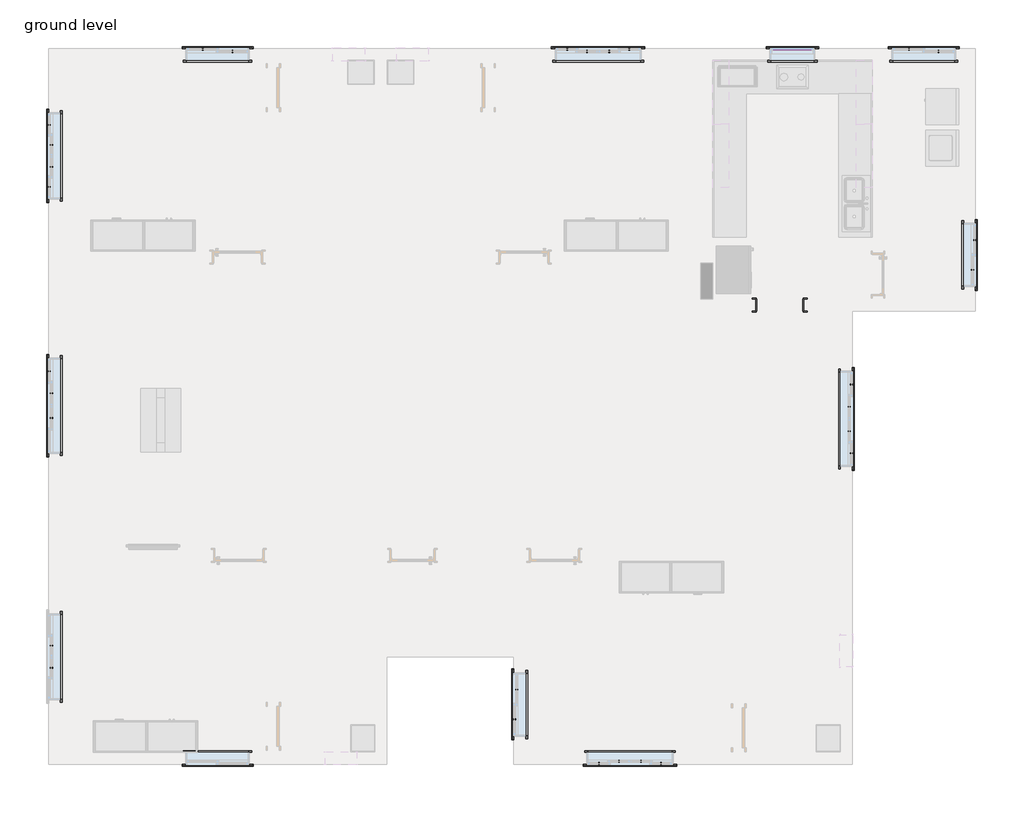
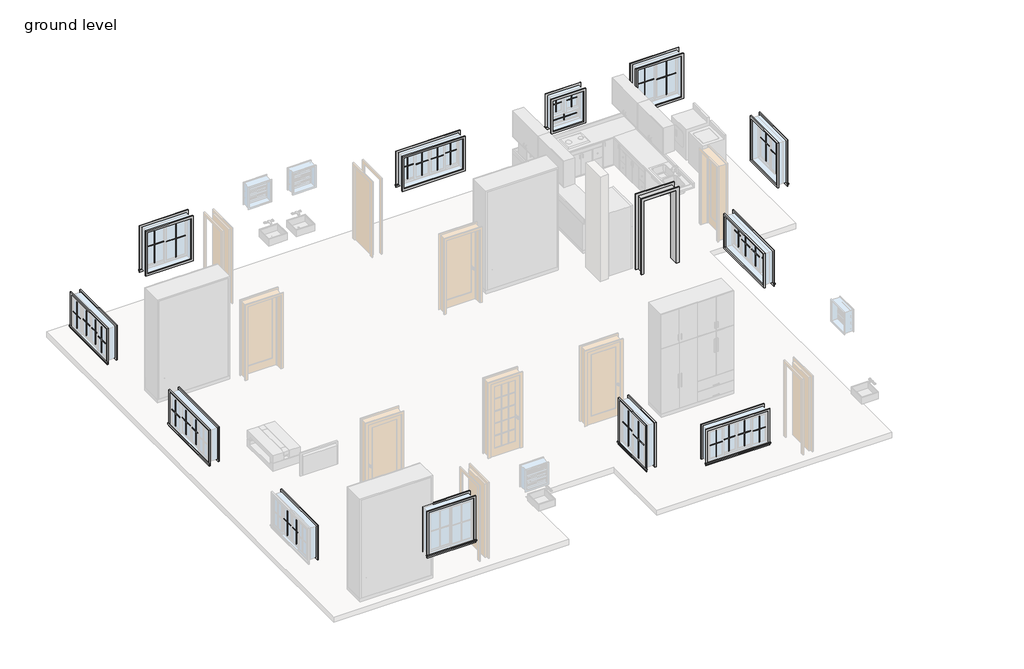
# One storey, part 2 of 2: 56 proxies.
"""IFC4 building model written with IfcOpenShell, lengths in millimetres."""

from ifc_helpers import new_model, si_unit, origin, place, context, project, spatial, transform, mapped, element, save
from components import muntin_pattern_2x2_muntin_pattern_2x2_6186d23a, muntin_pattern_2x2_muntin_pattern_2x2_31a16349, muntin_pattern_2x2_muntin_pattern_2x2_cf37b409, muntin_pattern_2x2_muntin_pattern_2x2_78ce0566, muntin_pattern_2x2_muntin_pattern_2x2_27bf4e5b, muntin_pattern_2x2_muntin_pattern_2x2_8320156c, proxy_e9bf662a, trim_window_exterior_flat_with_sill_c3f87112, trim_window_exterior_flat_with_sill_3c945769, trim_window_exterior_flat_with_sill_7cfdd449, trim_window_exterior_flat_with_sill_41619996, trim_window_interior_flat_picture_frame_1c33fa8a, trim_window_interior_flat_picture_frame_0edfbaa2, trim_window_interior_flat_picture_frame_f1e0b15b, trim_window_interior_flat_picture_frame_51c85655

model = new_model("IFC4")

# Units and contexts
model_context = context("Model", 3, world=origin())
ifc_project = project(units=[si_unit("LENGTHUNIT", "METRE", prefix="MILLI")], contexts=[model_context])

# Site, building, storey
site = spatial("IfcSite", under=ifc_project)
building = spatial("IfcBuilding", under=site)
storey = spatial("IfcBuildingStorey", under=building, Name="ground level", Elevation=609.6)

# Proxies
placement = place(None, origin())
muntin_pattern_2x2_muntin_pattern_2x2_shape = muntin_pattern_2x2_muntin_pattern_2x2_6186d23a(model_context)
element("IfcBuildingElementProxy", 1, Name="Muntin Pattern_2x2 : Muntin Pattern_2x2", ObjectType="Muntin Pattern_2x2 : Muntin Pattern_2x2", at=placement, inside=storey, context=model_context, shape_type="MappedRepresentation", body=[
    mapped(muntin_pattern_2x2_muntin_pattern_2x2_shape, transform((1905.0010838, 7064.4410813, 1606.55), x_axis=(1.0, 0.0, 0.0), y_axis=(0.0, 1.0, 0.0), z_axis=(0.0, 0.0, 1.0))),
])
element("IfcBuildingElementProxy", 2, Name="Muntin Pattern_2x2 : Muntin Pattern_2x2", ObjectType="Muntin Pattern_2x2 : Muntin Pattern_2x2", at=placement, inside=storey, context=model_context, shape_type="MappedRepresentation", body=[
    mapped(muntin_pattern_2x2_muntin_pattern_2x2_shape, transform((2286.0010838, 7019.9910813, 1606.55), x_axis=(1.0, 0.0, 0.0), y_axis=(0.0, 1.0, 0.0), z_axis=(0.0, 0.0, 1.0))),
])
element("IfcBuildingElementProxy", 3, Name="Muntin Pattern_2x2 : Muntin Pattern_2x2", ObjectType="Muntin Pattern_2x2 : Muntin Pattern_2x2", at=placement, inside=storey, context=model_context, shape_type="MappedRepresentation", body=[
    mapped(muntin_pattern_2x2_muntin_pattern_2x2_shape, transform((2711.4510838, 7019.9910813, 1606.55), x_axis=(1.0, 0.0, 0.0), y_axis=(0.0, 1.0, 0.0), z_axis=(0.0, 0.0, 1.0))),
])
element("IfcBuildingElementProxy", 4, Name="Muntin Pattern_2x2 : Muntin Pattern_2x2", ObjectType="Muntin Pattern_2x2 : Muntin Pattern_2x2", at=placement, inside=storey, context=model_context, shape_type="MappedRepresentation", body=[
    mapped(muntin_pattern_2x2_muntin_pattern_2x2_shape, transform((3092.4510838, 7064.4410813, 1606.55), x_axis=(1.0, 0.0, 0.0), y_axis=(0.0, 1.0, 0.0), z_axis=(0.0, 0.0, 1.0))),
])
element("IfcBuildingElementProxy", 5, Name="Muntin Pattern_2x2 : Muntin Pattern_2x2", ObjectType="Muntin Pattern_2x2 : Muntin Pattern_2x2", at=placement, inside=storey, context=model_context, shape_type="MappedRepresentation", body=[
    mapped(muntin_pattern_2x2_muntin_pattern_2x2_shape, transform((3702.0510838, -6632.5089187, 1606.55), x_axis=(-1.0, 0.0, 0.0), y_axis=(0.0, -1.0, 0.0), z_axis=(0.0, 0.0, 1.0))),
])
element("IfcBuildingElementProxy", 6, Name="Muntin Pattern_2x2 : Muntin Pattern_2x2", ObjectType="Muntin Pattern_2x2 : Muntin Pattern_2x2", at=placement, inside=storey, context=model_context, shape_type="MappedRepresentation", body=[
    mapped(muntin_pattern_2x2_muntin_pattern_2x2_shape, transform((3321.0510838, -6588.0589187, 1606.55), x_axis=(-1.0, 0.0, 0.0), y_axis=(0.0, -1.0, 0.0), z_axis=(0.0, 0.0, 1.0))),
])
element("IfcBuildingElementProxy", 7, Name="Muntin Pattern_2x2 : Muntin Pattern_2x2", ObjectType="Muntin Pattern_2x2 : Muntin Pattern_2x2", at=placement, inside=storey, context=model_context, shape_type="MappedRepresentation", body=[
    mapped(muntin_pattern_2x2_muntin_pattern_2x2_shape, transform((2895.6010838, -6588.0589187, 1606.55), x_axis=(-1.0, 0.0, 0.0), y_axis=(0.0, -1.0, 0.0), z_axis=(0.0, 0.0, 1.0))),
])
element("IfcBuildingElementProxy", 8, Name="Muntin Pattern_2x2 : Muntin Pattern_2x2", ObjectType="Muntin Pattern_2x2 : Muntin Pattern_2x2", at=placement, inside=storey, context=model_context, shape_type="MappedRepresentation", body=[
    mapped(muntin_pattern_2x2_muntin_pattern_2x2_shape, transform((2514.6010838, -6632.5089187, 1606.55), x_axis=(-1.0, 0.0, 0.0), y_axis=(0.0, -1.0, 0.0), z_axis=(0.0, 0.0, 1.0))),
])
element("IfcBuildingElementProxy", 9, Name="Muntin Pattern_2x2 : Muntin Pattern_2x2", ObjectType="Muntin Pattern_2x2 : Muntin Pattern_2x2", at=placement, inside=storey, context=model_context, shape_type="MappedRepresentation", body=[
    mapped(muntin_pattern_2x2_muntin_pattern_2x2_shape, transform((-8020.0489162, 4422.8410813, 1606.55), x_axis=(0.0, 1.0, 0.0), y_axis=(-1.0, 0.0, 0.0), z_axis=(0.0, 0.0, 1.0))),
])
element("IfcBuildingElementProxy", 10, Name="Muntin Pattern_2x2 : Muntin Pattern_2x2", ObjectType="Muntin Pattern_2x2 : Muntin Pattern_2x2", at=placement, inside=storey, context=model_context, shape_type="MappedRepresentation", body=[
    mapped(muntin_pattern_2x2_muntin_pattern_2x2_shape, transform((-7975.5989162, 4803.8410813, 1606.55), x_axis=(0.0, 1.0, 0.0), y_axis=(-1.0, 0.0, 0.0), z_axis=(0.0, 0.0, 1.0))),
])
element("IfcBuildingElementProxy", 11, Name="Muntin Pattern_2x2 : Muntin Pattern_2x2", ObjectType="Muntin Pattern_2x2 : Muntin Pattern_2x2", at=placement, inside=storey, context=model_context, shape_type="MappedRepresentation", body=[
    mapped(muntin_pattern_2x2_muntin_pattern_2x2_shape, transform((-7975.5989162, 5229.2910813, 1606.55), x_axis=(0.0, 1.0, 0.0), y_axis=(-1.0, 0.0, 0.0), z_axis=(0.0, 0.0, 1.0))),
])
element("IfcBuildingElementProxy", 12, Name="Muntin Pattern_2x2 : Muntin Pattern_2x2", ObjectType="Muntin Pattern_2x2 : Muntin Pattern_2x2", at=placement, inside=storey, context=model_context, shape_type="MappedRepresentation", body=[
    mapped(muntin_pattern_2x2_muntin_pattern_2x2_shape, transform((-8020.0489162, 5610.2910813, 1606.55), x_axis=(0.0, 1.0, 0.0), y_axis=(-1.0, 0.0, 0.0), z_axis=(0.0, 0.0, 1.0))),
])
element("IfcBuildingElementProxy", 13, Name="Muntin Pattern_2x2 : Muntin Pattern_2x2", ObjectType="Muntin Pattern_2x2 : Muntin Pattern_2x2", at=placement, inside=storey, context=model_context, shape_type="MappedRepresentation", body=[
    mapped(muntin_pattern_2x2_muntin_pattern_2x2_shape, transform((-7975.5989162, -4797.3589187, 1606.55), x_axis=(0.0, 1.0, 0.0), y_axis=(-1.0, 0.0, 0.0), z_axis=(0.0, 0.0, 1.0))),
])
element("IfcBuildingElementProxy", 14, Name="Muntin Pattern_2x2 : Muntin Pattern_2x2", ObjectType="Muntin Pattern_2x2 : Muntin Pattern_2x2", at=placement, inside=storey, context=model_context, shape_type="MappedRepresentation", body=[
    mapped(muntin_pattern_2x2_muntin_pattern_2x2_shape, transform((-7975.5989162, -4371.9089187, 1606.55), x_axis=(0.0, 1.0, 0.0), y_axis=(-1.0, 0.0, 0.0), z_axis=(0.0, 0.0, 1.0))),
])
muntin_pattern_2x2_muntin_pattern_2x2_2_shape = muntin_pattern_2x2_muntin_pattern_2x2_31a16349(model_context)
element("IfcBuildingElementProxy", 15, Name="Muntin Pattern_2x2 : Muntin Pattern_2x2", ObjectType="Muntin Pattern_2x2 : Muntin Pattern_2x2", at=placement, inside=storey, context=model_context, shape_type="MappedRepresentation", body=[
    mapped(muntin_pattern_2x2_muntin_pattern_2x2_2_shape, transform((-7975.5989162, -6.2839187, 1606.55), x_axis=(0.0, 1.0, 0.0), y_axis=(-1.0, 0.0, 0.0), z_axis=(0.0, 0.0, 1.0))),
])
element("IfcBuildingElementProxy", 16, Name="Muntin Pattern_2x2 : Muntin Pattern_2x2", ObjectType="Muntin Pattern_2x2 : Muntin Pattern_2x2", at=placement, inside=storey, context=model_context, shape_type="MappedRepresentation", body=[
    mapped(muntin_pattern_2x2_muntin_pattern_2x2_2_shape, transform((-7975.5989162, 463.6160813, 1606.55), x_axis=(0.0, 1.0, 0.0), y_axis=(-1.0, 0.0, 0.0), z_axis=(0.0, 0.0, 1.0))),
])
element("IfcBuildingElementProxy", 17, Name="Muntin Pattern_2x2 : Muntin Pattern_2x2", ObjectType="Muntin Pattern_2x2 : Muntin Pattern_2x2", at=placement, inside=storey, context=model_context, shape_type="MappedRepresentation", body=[
    mapped(muntin_pattern_2x2_muntin_pattern_2x2_2_shape, transform((-8020.0489162, 889.0660813, 1606.55), x_axis=(0.0, 1.0, 0.0), y_axis=(-1.0, 0.0, 0.0), z_axis=(0.0, 0.0, 1.0))),
])
element("IfcBuildingElementProxy", 18, Name="Muntin Pattern_2x2 : Muntin Pattern_2x2", ObjectType="Muntin Pattern_2x2 : Muntin Pattern_2x2", at=placement, inside=storey, context=model_context, shape_type="MappedRepresentation", body=[
    mapped(muntin_pattern_2x2_muntin_pattern_2x2_2_shape, transform((7353.3010838, 635.0660813, 1606.55), x_axis=(0.0, -1.0, 0.0), y_axis=(1.0, 0.0, 0.0), z_axis=(0.0, 0.0, 1.0))),
])
element("IfcBuildingElementProxy", 19, Name="Muntin Pattern_2x2 : Muntin Pattern_2x2", ObjectType="Muntin Pattern_2x2 : Muntin Pattern_2x2", at=placement, inside=storey, context=model_context, shape_type="MappedRepresentation", body=[
    mapped(muntin_pattern_2x2_muntin_pattern_2x2_2_shape, transform((7308.8510838, 209.6160813, 1606.55), x_axis=(0.0, -1.0, 0.0), y_axis=(1.0, 0.0, 0.0), z_axis=(0.0, 0.0, 1.0))),
])
element("IfcBuildingElementProxy", 20, Name="Muntin Pattern_2x2 : Muntin Pattern_2x2", ObjectType="Muntin Pattern_2x2 : Muntin Pattern_2x2", at=placement, inside=storey, context=model_context, shape_type="MappedRepresentation", body=[
    mapped(muntin_pattern_2x2_muntin_pattern_2x2_2_shape, transform((7308.8510838, -260.2839187, 1606.55), x_axis=(0.0, -1.0, 0.0), y_axis=(1.0, 0.0, 0.0), z_axis=(0.0, 0.0, 1.0))),
])
element("IfcBuildingElementProxy", 21, Name="Muntin Pattern_2x2 : Muntin Pattern_2x2", ObjectType="Muntin Pattern_2x2 : Muntin Pattern_2x2", at=placement, inside=storey, context=model_context, shape_type="MappedRepresentation", body=[
    mapped(muntin_pattern_2x2_muntin_pattern_2x2_2_shape, transform((7353.3010838, -685.7339187, 1606.55), x_axis=(0.0, -1.0, 0.0), y_axis=(1.0, 0.0, 0.0), z_axis=(0.0, 0.0, 1.0))),
])
muntin_pattern_2x2_muntin_pattern_2x2_3_shape = muntin_pattern_2x2_muntin_pattern_2x2_cf37b409(model_context)
element("IfcBuildingElementProxy", 22, Name="Muntin Pattern_2x2 : Muntin Pattern_2x2", ObjectType="Muntin Pattern_2x2 : Muntin Pattern_2x2", at=placement, inside=storey, context=model_context, shape_type="MappedRepresentation", body=[
    mapped(muntin_pattern_2x2_muntin_pattern_2x2_3_shape, transform((939.8010838, -5214.8714187, 1606.55), x_axis=(0.0, 1.0, 0.0), y_axis=(-1.0, 0.0, 0.0), z_axis=(0.0, 0.0, 1.0))),
])
element("IfcBuildingElementProxy", 23, Name="Muntin Pattern_2x2 : Muntin Pattern_2x2", ObjectType="Muntin Pattern_2x2 : Muntin Pattern_2x2", at=placement, inside=storey, context=model_context, shape_type="MappedRepresentation", body=[
    mapped(muntin_pattern_2x2_muntin_pattern_2x2_3_shape, transform((895.3510838, -5783.1964187, 1606.55), x_axis=(0.0, 1.0, 0.0), y_axis=(-1.0, 0.0, 0.0), z_axis=(0.0, 0.0, 1.0))),
])
element("IfcBuildingElementProxy", 24, Name="Muntin Pattern_2x2 : Muntin Pattern_2x2", ObjectType="Muntin Pattern_2x2 : Muntin Pattern_2x2", at=placement, inside=storey, context=model_context, shape_type="MappedRepresentation", body=[
    mapped(muntin_pattern_2x2_muntin_pattern_2x2_3_shape, transform((9018.5885838, 7019.9910813, 1606.55), x_axis=(1.0, 0.0, 0.0), y_axis=(0.0, 1.0, 0.0), z_axis=(0.0, 0.0, 1.0))),
])
element("IfcBuildingElementProxy", 25, Name="Muntin Pattern_2x2 : Muntin Pattern_2x2", ObjectType="Muntin Pattern_2x2 : Muntin Pattern_2x2", at=placement, inside=storey, context=model_context, shape_type="MappedRepresentation", body=[
    mapped(muntin_pattern_2x2_muntin_pattern_2x2_3_shape, transform((8450.2635838, 7064.4410813, 1606.55), x_axis=(1.0, 0.0, 0.0), y_axis=(0.0, 1.0, 0.0), z_axis=(0.0, 0.0, 1.0))),
])
element("IfcBuildingElementProxy", 26, Name="Muntin Pattern_2x2 : Muntin Pattern_2x2", ObjectType="Muntin Pattern_2x2 : Muntin Pattern_2x2", at=placement, inside=storey, context=model_context, shape_type="MappedRepresentation", body=[
    mapped(muntin_pattern_2x2_muntin_pattern_2x2_3_shape, transform((9671.3144662, 2832.6186041, 1606.55), x_axis=(0.0, -1.0, 0.0), y_axis=(1.0, 0.0, 0.0), z_axis=(0.0, 0.0, 1.0))),
])
element("IfcBuildingElementProxy", 27, Name="Muntin Pattern_2x2 : Muntin Pattern_2x2", ObjectType="Muntin Pattern_2x2 : Muntin Pattern_2x2", at=placement, inside=storey, context=model_context, shape_type="MappedRepresentation", body=[
    mapped(muntin_pattern_2x2_muntin_pattern_2x2_3_shape, transform((9715.7644662, 3400.9436041, 1606.55), x_axis=(0.0, -1.0, 0.0), y_axis=(1.0, 0.0, 0.0), z_axis=(0.0, 0.0, 1.0))),
])
element("IfcBuildingElementProxy", 28, Name="Muntin Pattern_2x2 : Muntin Pattern_2x2", ObjectType="Muntin Pattern_2x2 : Muntin Pattern_2x2", at=placement, inside=storey, context=model_context, shape_type="MappedRepresentation", body=[
    mapped(muntin_pattern_2x2_muntin_pattern_2x2_3_shape, transform((-4506.9114162, 7019.9910813, 1606.55), x_axis=(1.0, 0.0, 0.0), y_axis=(0.0, 1.0, 0.0), z_axis=(0.0, 0.0, 1.0))),
])
element("IfcBuildingElementProxy", 29, Name="Muntin Pattern_2x2 : Muntin Pattern_2x2", ObjectType="Muntin Pattern_2x2 : Muntin Pattern_2x2", at=placement, inside=storey, context=model_context, shape_type="MappedRepresentation", body=[
    mapped(muntin_pattern_2x2_muntin_pattern_2x2_3_shape, transform((-5075.2364162, 7064.4410813, 1606.55), x_axis=(1.0, 0.0, 0.0), y_axis=(0.0, 1.0, 0.0), z_axis=(0.0, 0.0, 1.0))),
])
muntin_pattern_2x2_muntin_pattern_2x2_4_shape = muntin_pattern_2x2_muntin_pattern_2x2_78ce0566(model_context)
element("IfcBuildingElementProxy", 30, Name="Muntin Pattern_2x2 : Muntin Pattern_2x2", ObjectType="Muntin Pattern_2x2 : Muntin Pattern_2x2", at=placement, inside=storey, context=model_context, shape_type="MappedRepresentation", body=[
    mapped(muntin_pattern_2x2_muntin_pattern_2x2_4_shape, transform((6005.5135838, 7064.4410813, 2127.25), x_axis=(1.0, 0.0, 0.0), y_axis=(0.0, 1.0, 0.0), z_axis=(0.0, 0.0, 1.0))),
])
muntin_pattern_2x2_muntin_pattern_2x2_5_shape = muntin_pattern_2x2_muntin_pattern_2x2_27bf4e5b(model_context)
element("IfcBuildingElementProxy", 31, Name="Muntin Pattern_2x2 : Muntin Pattern_2x2", ObjectType="Muntin Pattern_2x2 : Muntin Pattern_2x2", at=placement, inside=storey, context=model_context, shape_type="MappedRepresentation", body=[
    mapped(muntin_pattern_2x2_muntin_pattern_2x2_5_shape, transform((6434.1385838, 7064.4410813, 2127.25), x_axis=(-1.0, 0.0, 0.0), y_axis=(0.0, -1.0, 0.0), z_axis=(0.0, 0.0, 1.0))),
])
muntin_pattern_2x2_muntin_pattern_2x2_6_shape = muntin_pattern_2x2_muntin_pattern_2x2_8320156c(model_context)
element("IfcBuildingElementProxy", 32, Name="Muntin Pattern_2x2 : Muntin Pattern_2x2", ObjectType="Muntin Pattern_2x2 : Muntin Pattern_2x2", at=placement, inside=storey, context=model_context, shape_type="MappedRepresentation", body=[
    mapped(muntin_pattern_2x2_muntin_pattern_2x2_6_shape, transform((6219.8260838, 7064.4410813, 1822.45), x_axis=(-1.0, 0.0, 0.0), y_axis=(0.0, -1.0, 0.0), z_axis=(0.0, 0.0, 1.0))),
])
proxy_shape = proxy_e9bf662a(model_context)
element("IfcBuildingElementProxy", 33, Name="Passage Opening-Cased : 36\" x 84\"", ObjectType="Passage Opening-Cased : 36\" x 84\"", at=placement, inside=storey, context=model_context, shape_type="MappedRepresentation", body=[
    mapped(proxy_shape, transform((5970.337427, 2159.0660813, 609.6), x_axis=(-1.0, 0.0, 0.0), y_axis=(0.0, -1.0, 0.0), z_axis=(0.0, 0.0, 1.0))),
])
trim_window_exterior_flat_with_sill_shape = trim_window_exterior_flat_with_sill_c3f87112(model_context)
element("IfcBuildingElementProxy", 34, Name="Trim-Window-Exterior-Flat : with Sill", ObjectType="Trim-Window-Exterior-Flat : with Sill", at=placement, inside=storey, context=model_context, shape_type="MappedRepresentation", body=[
    mapped(trim_window_exterior_flat_with_sill_shape, transform((2498.7260838, 7073.9660813, 2438.4), x_axis=(-1.0, 0.0, 0.0), y_axis=(0.0, 0.0, 1.0), z_axis=(0.0, 1.0, 0.0))),
])
element("IfcBuildingElementProxy", 35, Name="Trim-Window-Exterior-Flat : with Sill", ObjectType="Trim-Window-Exterior-Flat : with Sill", at=placement, inside=storey, context=model_context, shape_type="MappedRepresentation", body=[
    mapped(trim_window_exterior_flat_with_sill_shape, transform((3108.3260838, -6642.0339187, 2438.4), x_axis=(1.0, 0.0, 0.0), y_axis=(0.0, 0.0, 1.0), z_axis=(0.0, -1.0, 0.0))),
])
element("IfcBuildingElementProxy", 36, Name="Trim-Window-Exterior-Flat : with Sill", ObjectType="Trim-Window-Exterior-Flat : with Sill", at=placement, inside=storey, context=model_context, shape_type="MappedRepresentation", body=[
    mapped(trim_window_exterior_flat_with_sill_shape, transform((-8029.5739162, 5016.5660813, 2438.4), x_axis=(0.0, -1.0, 0.0), y_axis=(0.0, 0.0, 1.0), z_axis=(-1.0, 0.0, 0.0))),
])
trim_window_exterior_flat_with_sill_2_shape = trim_window_exterior_flat_with_sill_3c945769(model_context)
element("IfcBuildingElementProxy", 37, Name="Trim-Window-Exterior-Flat : with Sill", ObjectType="Trim-Window-Exterior-Flat : with Sill", at=placement, inside=storey, context=model_context, shape_type="MappedRepresentation", body=[
    mapped(trim_window_exterior_flat_with_sill_2_shape, transform((-8029.5739162, 228.6660813, 2438.4), x_axis=(0.0, -1.0, 0.0), y_axis=(0.0, 0.0, 1.0), z_axis=(-1.0, 0.0, 0.0))),
])
element("IfcBuildingElementProxy", 38, Name="Trim-Window-Exterior-Flat : with Sill", ObjectType="Trim-Window-Exterior-Flat : with Sill", at=placement, inside=storey, context=model_context, shape_type="MappedRepresentation", body=[
    mapped(trim_window_exterior_flat_with_sill_2_shape, transform((7362.8260838, -25.3339187, 2438.4), x_axis=(0.0, 1.0, 0.0), y_axis=(0.0, 0.0, 1.0), z_axis=(1.0, 0.0, 0.0))),
])
trim_window_exterior_flat_with_sill_3_shape = trim_window_exterior_flat_with_sill_7cfdd449(model_context)
element("IfcBuildingElementProxy", 39, Name="Trim-Window-Exterior-Flat : with Sill", ObjectType="Trim-Window-Exterior-Flat : with Sill", at=placement, inside=storey, context=model_context, shape_type="MappedRepresentation", body=[
    mapped(trim_window_exterior_flat_with_sill_3_shape, transform((885.8260838, -5499.0339187, 2743.2), x_axis=(0.0, -1.0, 0.0), y_axis=(0.0, 0.0, 1.0), z_axis=(-1.0, 0.0, 0.0))),
])
element("IfcBuildingElementProxy", 40, Name="Trim-Window-Exterior-Flat : with Sill", ObjectType="Trim-Window-Exterior-Flat : with Sill", at=placement, inside=storey, context=model_context, shape_type="MappedRepresentation", body=[
    mapped(trim_window_exterior_flat_with_sill_3_shape, transform((8734.4260838, 7073.9660813, 2743.2), x_axis=(-1.0, 0.0, 0.0), y_axis=(0.0, 0.0, 1.0), z_axis=(0.0, 1.0, 0.0))),
])
element("IfcBuildingElementProxy", 41, Name="Trim-Window-Exterior-Flat : with Sill", ObjectType="Trim-Window-Exterior-Flat : with Sill", at=placement, inside=storey, context=model_context, shape_type="MappedRepresentation", body=[
    mapped(trim_window_exterior_flat_with_sill_3_shape, transform((9725.2894662, 3116.7811041, 2743.2), x_axis=(0.0, 1.0, 0.0), y_axis=(0.0, 0.0, 1.0), z_axis=(1.0, 0.0, 0.0))),
])
element("IfcBuildingElementProxy", 42, Name="Trim-Window-Exterior-Flat : with Sill", ObjectType="Trim-Window-Exterior-Flat : with Sill", at=placement, inside=storey, context=model_context, shape_type="MappedRepresentation", body=[
    mapped(trim_window_exterior_flat_with_sill_3_shape, transform((-4791.0739162, -6642.0339187, 2743.2), x_axis=(1.0, 0.0, 0.0), y_axis=(0.0, 0.0, 1.0), z_axis=(0.0, -1.0, 0.0))),
])
element("IfcBuildingElementProxy", 43, Name="Trim-Window-Exterior-Flat : with Sill", ObjectType="Trim-Window-Exterior-Flat : with Sill", at=placement, inside=storey, context=model_context, shape_type="MappedRepresentation", body=[
    mapped(trim_window_exterior_flat_with_sill_3_shape, transform((-4791.0739162, 7073.9660813, 2743.2), x_axis=(-1.0, 0.0, 0.0), y_axis=(0.0, 0.0, 1.0), z_axis=(0.0, 1.0, 0.0))),
])
trim_window_exterior_flat_with_sill_4_shape = trim_window_exterior_flat_with_sill_41619996(model_context)
element("IfcBuildingElementProxy", 44, Name="Trim-Window-Exterior-Flat : with Sill", ObjectType="Trim-Window-Exterior-Flat : with Sill", at=placement, inside=storey, context=model_context, shape_type="MappedRepresentation", body=[
    mapped(trim_window_exterior_flat_with_sill_4_shape, transform((6219.8260838, 7073.9660813, 2667.0), x_axis=(-1.0, 0.0, 0.0), y_axis=(0.0, 0.0, 1.0), z_axis=(0.0, 1.0, 0.0))),
])
trim_window_interior_flat_picture_frame_shape = trim_window_interior_flat_picture_frame_1c33fa8a(model_context)
element("IfcBuildingElementProxy", 45, Name="Trim-Window-Interior-Flat : Picture Frame", ObjectType="Trim-Window-Interior-Flat : Picture Frame", at=placement, inside=storey, context=model_context, shape_type="MappedRepresentation", body=[
    mapped(trim_window_interior_flat_picture_frame_shape, transform((2498.7260838, 6845.3660813, 2438.4), x_axis=(1.0, 0.0, 0.0), y_axis=(0.0, 0.0, 1.0), z_axis=(0.0, -1.0, 0.0))),
])
element("IfcBuildingElementProxy", 46, Name="Trim-Window-Interior-Flat : Picture Frame", ObjectType="Trim-Window-Interior-Flat : Picture Frame", at=placement, inside=storey, context=model_context, shape_type="MappedRepresentation", body=[
    mapped(trim_window_interior_flat_picture_frame_shape, transform((3108.3260838, -6413.4339187, 2438.4), x_axis=(-1.0, 0.0, 0.0), y_axis=(0.0, 0.0, 1.0), z_axis=(0.0, 1.0, 0.0))),
])
element("IfcBuildingElementProxy", 47, Name="Trim-Window-Interior-Flat : Picture Frame", ObjectType="Trim-Window-Interior-Flat : Picture Frame", at=placement, inside=storey, context=model_context, shape_type="MappedRepresentation", body=[
    mapped(trim_window_interior_flat_picture_frame_shape, transform((-7800.9739162, 5016.5660813, 2438.4), x_axis=(0.0, 1.0, 0.0), y_axis=(0.0, 0.0, 1.0), z_axis=(1.0, 0.0, 0.0))),
])
element("IfcBuildingElementProxy", 48, Name="Trim-Window-Interior-Flat : Picture Frame", ObjectType="Trim-Window-Interior-Flat : Picture Frame", at=placement, inside=storey, context=model_context, shape_type="MappedRepresentation", body=[
    mapped(trim_window_interior_flat_picture_frame_shape, transform((-7800.9739162, -4584.6339187, 2438.4), x_axis=(0.0, 1.0, 0.0), y_axis=(0.0, 0.0, 1.0), z_axis=(1.0, 0.0, 0.0))),
])
trim_window_interior_flat_picture_frame_2_shape = trim_window_interior_flat_picture_frame_0edfbaa2(model_context)
element("IfcBuildingElementProxy", 49, Name="Trim-Window-Interior-Flat : Picture Frame", ObjectType="Trim-Window-Interior-Flat : Picture Frame", at=placement, inside=storey, context=model_context, shape_type="MappedRepresentation", body=[
    mapped(trim_window_interior_flat_picture_frame_2_shape, transform((-7800.9739162, 228.6660813, 2438.4), x_axis=(0.0, 1.0, 0.0), y_axis=(0.0, 0.0, 1.0), z_axis=(1.0, 0.0, 0.0))),
])
element("IfcBuildingElementProxy", 50, Name="Trim-Window-Interior-Flat : Picture Frame", ObjectType="Trim-Window-Interior-Flat : Picture Frame", at=placement, inside=storey, context=model_context, shape_type="MappedRepresentation", body=[
    mapped(trim_window_interior_flat_picture_frame_2_shape, transform((7134.2260838, -25.3339187, 2438.4), x_axis=(0.0, -1.0, 0.0), y_axis=(0.0, 0.0, 1.0), z_axis=(-1.0, 0.0, 0.0))),
])
trim_window_interior_flat_picture_frame_3_shape = trim_window_interior_flat_picture_frame_f1e0b15b(model_context)
element("IfcBuildingElementProxy", 51, Name="Trim-Window-Interior-Flat : Picture Frame", ObjectType="Trim-Window-Interior-Flat : Picture Frame", at=placement, inside=storey, context=model_context, shape_type="MappedRepresentation", body=[
    mapped(trim_window_interior_flat_picture_frame_3_shape, transform((1114.4260838, -5499.0339187, 2743.2), x_axis=(0.0, 1.0, 0.0), y_axis=(0.0, 0.0, 1.0), z_axis=(1.0, 0.0, 0.0))),
])
element("IfcBuildingElementProxy", 52, Name="Trim-Window-Interior-Flat : Picture Frame", ObjectType="Trim-Window-Interior-Flat : Picture Frame", at=placement, inside=storey, context=model_context, shape_type="MappedRepresentation", body=[
    mapped(trim_window_interior_flat_picture_frame_3_shape, transform((8734.4260838, 6845.3660813, 2743.2), x_axis=(1.0, 0.0, 0.0), y_axis=(0.0, 0.0, 1.0), z_axis=(0.0, -1.0, 0.0))),
])
element("IfcBuildingElementProxy", 53, Name="Trim-Window-Interior-Flat : Picture Frame", ObjectType="Trim-Window-Interior-Flat : Picture Frame", at=placement, inside=storey, context=model_context, shape_type="MappedRepresentation", body=[
    mapped(trim_window_interior_flat_picture_frame_3_shape, transform((9496.6894662, 3116.7811041, 2743.2), x_axis=(0.0, -1.0, 0.0), y_axis=(0.0, 0.0, 1.0), z_axis=(-1.0, 0.0, 0.0))),
])
element("IfcBuildingElementProxy", 54, Name="Trim-Window-Interior-Flat : Picture Frame", ObjectType="Trim-Window-Interior-Flat : Picture Frame", at=placement, inside=storey, context=model_context, shape_type="MappedRepresentation", body=[
    mapped(trim_window_interior_flat_picture_frame_3_shape, transform((-4791.0739162, -6413.4339187, 2743.2), x_axis=(-1.0, 0.0, 0.0), y_axis=(0.0, 0.0, 1.0), z_axis=(0.0, 1.0, 0.0))),
])
element("IfcBuildingElementProxy", 55, Name="Trim-Window-Interior-Flat : Picture Frame", ObjectType="Trim-Window-Interior-Flat : Picture Frame", at=placement, inside=storey, context=model_context, shape_type="MappedRepresentation", body=[
    mapped(trim_window_interior_flat_picture_frame_3_shape, transform((-4791.0739162, 6845.3660813, 2743.2), x_axis=(1.0, 0.0, 0.0), y_axis=(0.0, 0.0, 1.0), z_axis=(0.0, -1.0, 0.0))),
])
trim_window_interior_flat_picture_frame_4_shape = trim_window_interior_flat_picture_frame_51c85655(model_context)
element("IfcBuildingElementProxy", 56, Name="Trim-Window-Interior-Flat : Picture Frame", ObjectType="Trim-Window-Interior-Flat : Picture Frame", at=placement, inside=storey, context=model_context, shape_type="MappedRepresentation", body=[
    mapped(trim_window_interior_flat_picture_frame_4_shape, transform((6219.8260838, 6845.3660813, 2667.0), x_axis=(1.0, 0.0, 0.0), y_axis=(0.0, 0.0, 1.0), z_axis=(0.0, -1.0, 0.0))),
])

save(model, "model.ifc")

# Revit data of these elements
# Type "Muntin Pattern_2x2 : Muntin Pattern_2x2"
#   Width [instance default] = 4' - 0"
#   Thickness = 0' - 0 1/2"
#   Height [instance default] = 4' - 0"
#   Distance = 0' - 0 3/4"
#   Interior Material [instance default] = none
#   Exterior Material [instance default] = none
#   Default Elevation = 0
# Type "Passage Opening-Cased : 36\" x 84\""
#   Height = 7' - 0"
#   Trim Thickness = 0' - 0 3/4"
#   Trim Width = 0' - 3"
#   Width = 3' - 0"
#   Frame Material = Door - Frame
#   Default Elevation = 0
# Type "Trim-Window-Exterior-Flat : with Sill"
#   Trim Width = 0' - 2 1/4"
#   Trim Thickness_Picture Frame = 0' - 1 1/4"
#   Trim Thickness_with Sill = 0' - 0 3/4"
#   Sill Thickness = 0' - 1 1/4"
#   Opening Width [instance default] = 2' - 0"
#   Opening Height [instance default] = 3' - 0"
#   Default Elevation = 4' - 0"
#   Sill = yes
#   Picture Frame = no
#   Trim Material [instance default] = none
# Type "Trim-Window-Interior-Flat : Picture Frame"
#   Trim Thickness_Picture Frame = 0' - 1 1/4"
#   Trim Width = 0' - 2 1/4"
#   Trim Thickness_with Sill = 0' - 0 3/4"
#   Sill Thickness = 0' - 1 1/4"
#   Opening Width [instance default] = 2' - 0"
#   Opening Height [instance default] = 3' - 0"
#   Default Elevation = 4' - 0"
#   Sill = no
#   Picture Frame = yes
#   Trim Material [instance default] = none
# Elements 1, 2, 3, 4, 5, 6, 7, 8, 9, 10, 11, 12, 13, 14 (IfcBuildingElementProxy, "Muntin Pattern_2x2 : Muntin Pattern_2x2")
#   Width = 1' - 1 1/4"
#   Height = 2' - 6 1/4"
#   Interior Material = Wood - Stained
#   Exterior Material = Clad - White
#   Phase Created = New Construction
#   Materials on its faces: "Clad - White", "Wood - Stained"
# Elements 15, 16, 17, 18, 19, 20, 21 (IfcBuildingElementProxy, "Muntin Pattern_2x2 : Muntin Pattern_2x2")
#   Width = 1' - 3"
#   Height = 2' - 6 1/4"
#   Interior Material = Wood - Stained
#   Exterior Material = Clad - White
#   Phase Created = New Construction
#   Materials on its faces: "Clad - White", "Wood - Stained"
# Elements 22, 23, 24, 25, 26, 27, 28, 29 (IfcBuildingElementProxy, "Muntin Pattern_2x2 : Muntin Pattern_2x2")
#   Width = 1' - 8 5/8"
#   Height = 3' - 6 1/4"
#   Interior Material = Wood - Stained
#   Exterior Material = Clad - White
#   Phase Created = New Construction
#   Materials on its faces: "Clad - White", "Wood - Stained"
# Elements 30, 31 (IfcBuildingElementProxy, "Muntin Pattern_2x2 : Muntin Pattern_2x2")
#   Width = 0' - 11 5/8"
#   Height = 1' - 6 1/2"
#   Interior Material = Wood - Stained
#   Exterior Material = Clad - White
#   Phase Created = New Construction
#   Materials on its faces: "Clad - White", "Wood - Stained"
# Element 32 (IfcBuildingElementProxy, "Muntin Pattern_2x2 : Muntin Pattern_2x2")
#   Width = 2' - 4 1/2"
#   Height = 0' - 6 1/2"
#   Interior Material = Wood - Stained
#   Exterior Material = Clad - White
#   Phase Created = New Construction
#   Materials on its faces: "Clad - White", "Wood - Stained"
# Element 33 (IfcBuildingElementProxy, "Passage Opening-Cased : 36\" x 84\"")
#   Phase Created = New Construction
#   Materials on its faces: "Door - Frame"
# Elements 34, 35, 36 (IfcBuildingElementProxy, "Trim-Window-Exterior-Flat : with Sill")
#   Opening Width = 5' - 5"
#   Opening Height = 3' - 0"
#   Trim Material = Clad - White
#   Phase Created = New Construction
#   Materials on its faces: "Clad - White"
# Elements 37, 38 (IfcBuildingElementProxy, "Trim-Window-Exterior-Flat : with Sill")
#   Opening Width = 6' - 0"
#   Opening Height = 3' - 0"
#   Trim Material = Clad - White
#   Phase Created = New Construction
#   Materials on its faces: "Clad - White"
# Elements 39, 40, 41, 42, 43 (IfcBuildingElementProxy, "Trim-Window-Exterior-Flat : with Sill")
#   Opening Width = 4' - 0"
#   Opening Height = 4' - 0"
#   Trim Material = Clad - White
#   Phase Created = New Construction
#   Materials on its faces: "Clad - White"
# Element 44 (IfcBuildingElementProxy, "Trim-Window-Exterior-Flat : with Sill")
#   Opening Width = 2' - 10"
#   Opening Height = 3' - 0"
#   Trim Material = Clad - White
#   Phase Created = New Construction
#   Materials on its faces: "Clad - White"
# Elements 45, 46, 47, 48 (IfcBuildingElementProxy, "Trim-Window-Interior-Flat : Picture Frame")
#   Opening Width = 5' - 5"
#   Opening Height = 3' - 0"
#   Trim Material = Wood - Stained
#   Phase Created = New Construction
#   Materials on its faces: "Wood - Stained"
# Elements 49, 50 (IfcBuildingElementProxy, "Trim-Window-Interior-Flat : Picture Frame")
#   Opening Width = 6' - 0"
#   Opening Height = 3' - 0"
#   Trim Material = Wood - Stained
#   Phase Created = New Construction
#   Materials on its faces: "Wood - Stained"
# Elements 51, 52, 53, 54, 55 (IfcBuildingElementProxy, "Trim-Window-Interior-Flat : Picture Frame")
#   Opening Width = 4' - 0"
#   Opening Height = 4' - 0"
#   Trim Material = Wood - Stained
#   Phase Created = New Construction
#   Materials on its faces: "Wood - Stained"
# Element 56 (IfcBuildingElementProxy, "Trim-Window-Interior-Flat : Picture Frame")
#   Opening Width = 2' - 10"
#   Opening Height = 3' - 0"
#   Trim Material = Wood - Stained
#   Phase Created = New Construction
#   Materials on its faces: "Wood - Stained"
# Materials
#   "Door - Frame": colour RGB 118 70 51, transparency 0, Cost = 0
#   "Clad - White": class "Wood", colour RGB 242 242 238, transparency 0, Cost = 0
#   "Wood - Stained": class "Wood", colour RGB 224 178 126, transparency 0, Cost = 0
